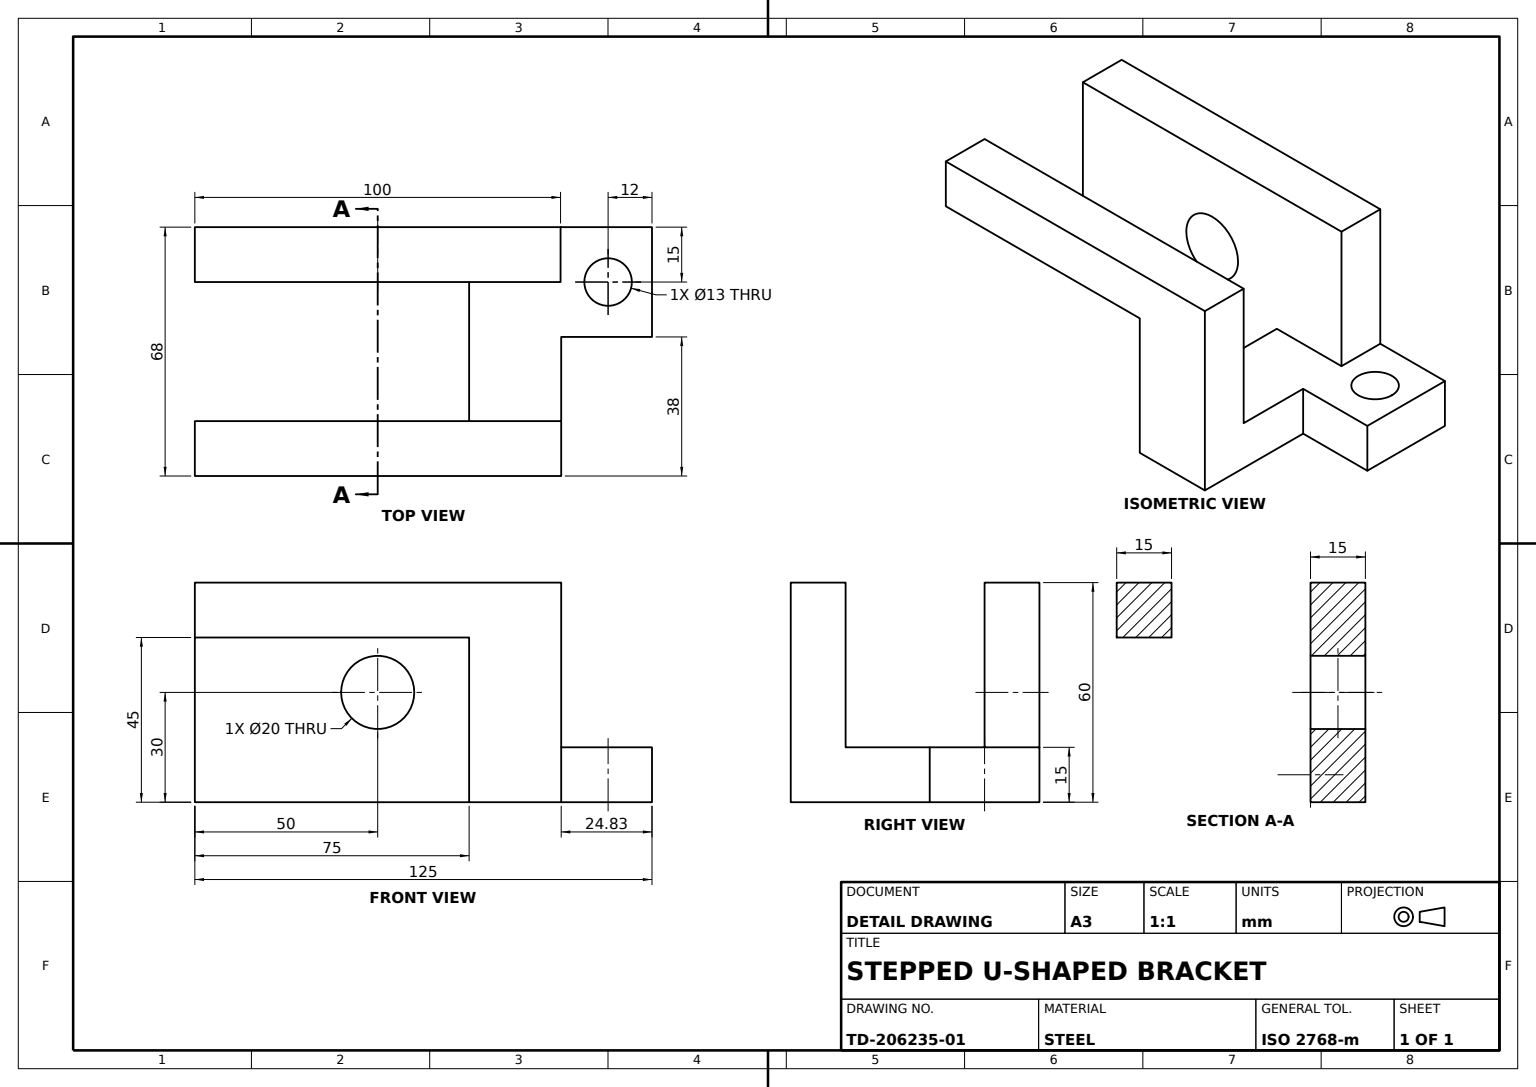
SolidWorks part; units mm, degrees
material "Plain Carbon Steel"
ref_plane "Front Plane" through (0, 0, 0) normal (0, 0, 1) x (1, 0, 0)
ref_plane "Top Plane" through (0, 0, 0) normal (0, 1, 0) x (1, 0, 0)
ref_plane "Right Plane" through (0, 0, 0) normal (1, 0, 0) x (0, 0, -1)
sketch "Base Plate Sketch" plane through (0, 0, 0) normal (0, 0, 1) x (1, 0, 0)
  line L1 (-50, -30) -> (50, -30)
  line L2 (-50, -30) -> (-50, 30)
  line L3 (-50, 30) -> (50, 30)
  line L4 (50, -30) -> (50, 30)
  point P0 (0, 0)
  dimension "D1" = 100
  dimension "D2" = 60
  dimension "D3" = 50
  dimension "D4" = 30
extrude "Base Plate" add sketch "Base Plate Sketch" along normal blind 15
sketch "Upright Block Sketch" plane through (0, 0, 0) normal (0, 0, -1) x (-1, 0, 0)
  line L0 (-25, -30) -> (-25, -15)
  line L1 (-25, -30) -> (-75, -30)
  line L2 (-25, -15) -> (-75, -15)
  line L3 (-75, -30) -> (-75, -15)
  line L4 (50, -30) -> (-50, -30) construction
  line L5 (-50, -30) -> (-50, 30) construction
  dimension "D1" = 50
  dimension "D2" = 25
  dimension "D3" = 15
extrude "Upright Block" add sketch "Upright Block Sketch" against normal blind 30
sketch "Side Wall Sketch" plane through (0, 0, 30) normal (0, 0, 1) x (1, 0, 0)
  line L0 (25, -30) -> (25, -15)
  line L1 (25, -30) -> (50.1744, -30)
  line L2 (25, -15) -> (50.1744, -15)
  line L3 (50.1744, -30) -> (50.1744, -15)
  line L4 (75, -15) -> (75, -30) construction
  dimension "D1" = 24.8256
extrude "Side Wall" add sketch "Side Wall Sketch" along normal blind 38
sketch "Lower Arm Sketch" plane through (0, -15, 0) normal (0, 1, 0) x (1, 0, 0)
  line L0 (25, -68) -> (25, -53)
  line L1 (25, -68) -> (50.1744, -68)
  line L2 (25, -53) -> (50.1744, -53)
  line L3 (50.1744, -68) -> (50.1744, -53)
  line L4 (25, -68) -> (25, -15) construction
  line L5 (50.1744, -68) -> (50.1744, -30) construction
  dimension "D1" = 15
extrude "Lower Arm" add sketch "Lower Arm Sketch" along normal blind 45
sketch "Upper Arm Sketch" plane through (25, 0, 0) normal (-1, 0, 0) x (0, 0, 1)
  line L0 (53, 30) -> (68, 30)
  line L1 (53, 30) -> (53, 15)
  line L2 (68, 30) -> (68, 15)
  line L3 (53, 15) -> (68, 15)
  dimension "D1" = 15
extrude "Upper Arm" add sketch "Upper Arm Sketch" along normal blind 75
sketch "Wall Hole Sketch" plane through (0, -15, 0) normal (0, 1, 0) x (1, 0, 0)
  line L0 (75, -30) -> (75, 0) construction
  line L1 (50, 0) -> (75, 0) construction
  circle A0 centre (63, -15) radius 6.5
  dimension "D1" = 12
  dimension "D2" = 13
  dimension "D3" = 15
extrude "Wall Through Hole" cut sketch "Wall Hole Sketch" against normal blind 75
sketch "Base Hole Sketch" plane through (0, 0, 15) normal (0, 0, 1) x (1, 0, 0)
  circle A0 centre (0, 0) radius 10
  dimension "D1" = 20
extrude "Base Through Hole" cut sketch "Base Hole Sketch" against normal blind 75
